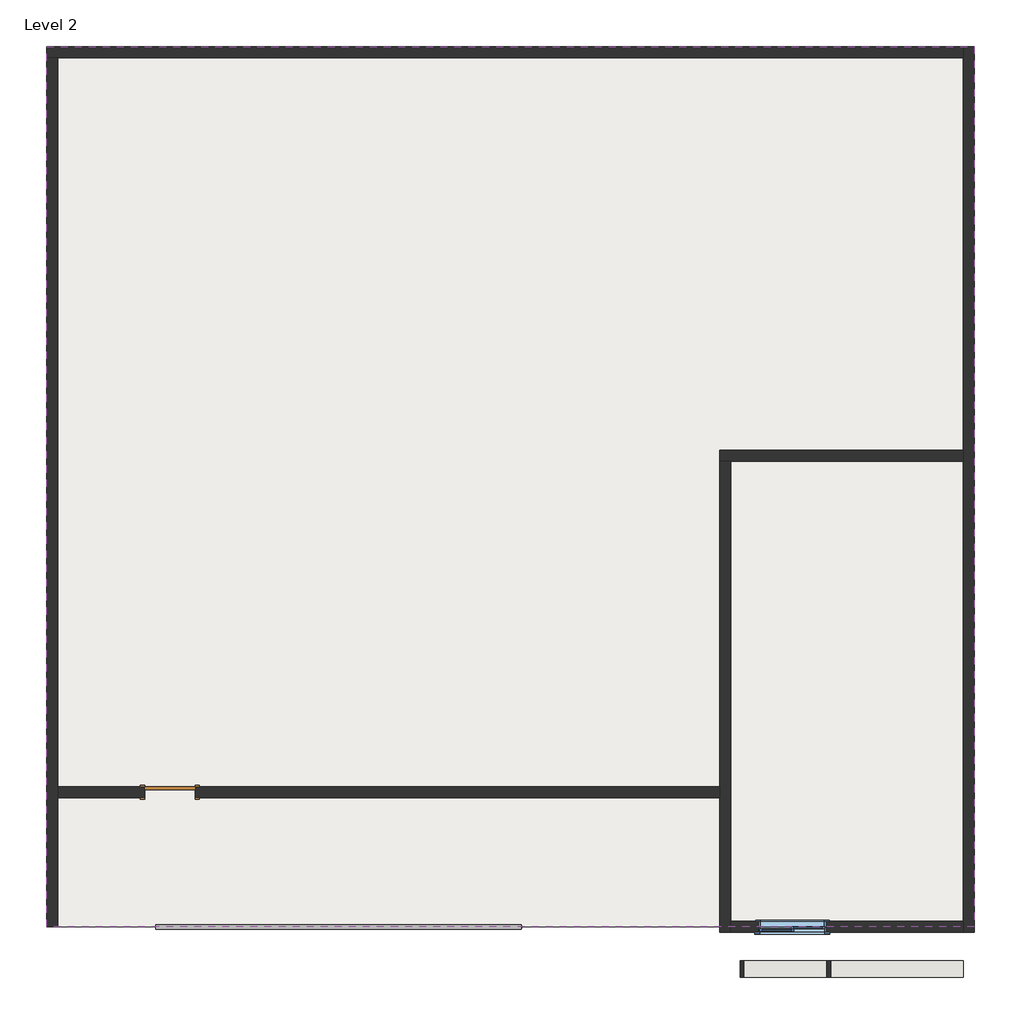
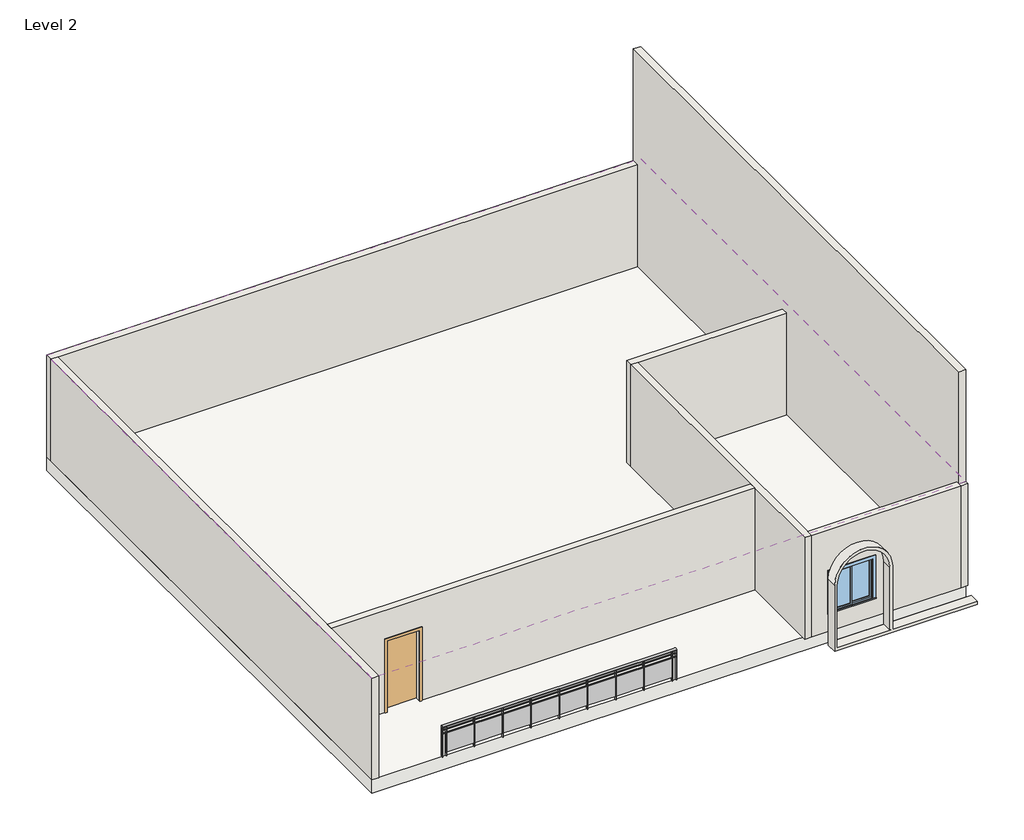
# One storey: 8 walls, 1 covering, 1 door, 1 railing, 1 slab, 1 window.
"""IFC4 building model written with IfcOpenShell, lengths in millimetres."""

from ifc_helpers import new_model, si_unit, point, frame, origin, place, context, project, spatial, polyline, ellipse_curve, trimmed, outline, extrude, faceted_brep, transform, mapped, element, save
from ifc_brep_helpers import plane_surface, extruded_surface, advanced_brep
from components import m_single_flush_0915_x_2134mm_727434cd, walls_5_walls_5_0e1fe4ca, window_deda82dd

model = new_model("IFC4")

# Units and contexts
model_context = context("Model", 3, world=origin())
ifc_project = project(units=[si_unit("LENGTHUNIT", "METRE", prefix="MILLI")], contexts=[model_context])

# Site, building, storey
site = spatial("IfcSite", under=ifc_project)
building = spatial("IfcBuilding", under=site)
storey = spatial("IfcBuildingStorey", under=building, Name="Level 2", Elevation=6096.0)

# Covering
placement = place(None, origin())
element("IfcCovering", 1, ObjectType="600 x 1200mm grid", at=placement, inside=storey, context=model_context, shape_type="SweptSolid", body=[
    extrude(outline(polyline([(-9031.8352527, 15360.4148445), (7778.3159626, 15360.4148445), (7778.3159626, -589.1851555), (-9031.8352527, -589.1851555), (-9031.8352527, 15360.4148445)])), frame((0.0, 0.0, 9144.0), z_axis=(0.0, 0.0, 1.0), x_axis=(1.0, 0.0, 0.0)), (0.0, 0.0, 1.0), 52.0),
])

# Door
m_single_flush_0915_x_2134mm_shape = m_single_flush_0915_x_2134mm_727434cd(model_context)
element("IfcDoor", 2, ObjectType="M_Single-Flush : 0915 x 2134mm", at=placement, inside=storey, context=model_context, shape_type="MappedRepresentation", body=[
    mapped(m_single_flush_0915_x_2134mm_shape, transform((-6798.2352527, 1849.2148445, 6096.0), x_axis=(-1.0, 0.0, 0.0), y_axis=(0.0, -1.0, 0.0), z_axis=(0.0, 0.0, 1.0))),
])

# Railing
element("IfcRailing", 3, ObjectType="Glass Panel - Bottom Fill", at=placement, inside=storey, context=model_context, shape_type="SolidModel", body=[
    advanced_brep(
    [(-7050.6352527, -549.7943903, 6996.0), (-7050.6352527, -629.7943903, 6996.0), (-429.4748459, -549.7943903, 6996.0), (-429.4748459, -629.7943903, 6996.0)],
    [
        (0, 1, ellipse_curve(frame((-7050.6352527, -589.7943903, 6996.0), z_axis=(-1.0, 0.0, 0.0), x_axis=(0.0, -1.0, 0.0)), 40.0, 30.0)),
        (1, 0, ellipse_curve(frame((-7050.6352527, -589.7943903, 6996.0), z_axis=(-1.0, 0.0, 0.0), x_axis=(0.0, -1.0, 0.0)), 40.0, 30.0)),
        (2, 3, ellipse_curve(frame((-429.4748459, -589.7943903, 6996.0), z_axis=(1.0, 0.0, 0.0), x_axis=(0.0, -1.0, 0.0)), 40.0, 30.0)),
        (3, 2, ellipse_curve(frame((-429.4748459, -589.7943903, 6996.0), z_axis=(1.0, 0.0, 0.0), x_axis=(0.0, -1.0, 0.0)), 40.0, 30.0)),
        (1, 3),
        (2, 0),
    ],
    [
        plane_surface(frame((-7050.6352527, -589.7943903, 6996.0), z_axis=(-1.0, 0.0, 0.0), x_axis=(0.0, 1.0, 0.0))),
        plane_surface(frame((-429.4748459, -589.7943903, 6996.0), z_axis=(1.0, 0.0, 0.0), x_axis=(0.0, 1.0, 0.0))),
        extruded_surface(trimmed(ellipse_curve(frame((-429.4748459, -589.7943903, 6996.0), z_axis=(-1.0, 0.0, 0.0), x_axis=(0.0, -1.0, 0.0)), 40.0, 30.0), [point((-429.4748459, -629.7943903, 6996.0))], [point((-429.4748459, -549.7943903, 6996.0))], True, "CARTESIAN"), (-6621.1604068, 0.0, 0.0), 6621.1604068),
        extruded_surface(trimmed(ellipse_curve(frame((-429.4748459, -589.7943903, 6996.0), z_axis=(-1.0, 0.0, 0.0), x_axis=(0.0, -1.0, 0.0)), 40.0, 30.0), [point((-429.4748459, -549.7943903, 6996.0))], [point((-429.4748459, -629.7943903, 6996.0))], True, "CARTESIAN"), (-6621.1604068, 0.0, 0.0), 6621.1604068),
    ],
    [
        (0, [[1, 2]]),
        (1, [[3, 4]]),
        (2, [[-2, 5, -3, 6]]),
        (3, [[-1, -6, -4, -5]]),
    ],
),
    extrude(outline(polyline([(-7050.6352527, -599.1851555), (-7050.6352527, -579.1851555), (-429.4748459, -579.1851555), (-429.4748459, -599.1851555), (-7050.6352527, -599.1851555)])), frame((0.0, 0.0, 6876.0), z_axis=(0.0, 0.0, 1.0), x_axis=(1.0, 0.0, 0.0)), (0.0, 0.0, 1.0), 20.0),
    extrude(outline(polyline([(-7050.6352527, -599.1851555), (-7050.6352527, -579.1851555), (-429.4748459, -579.1851555), (-429.4748459, -599.1851555), (-7050.6352527, -599.1851555)])), frame((0.0, 0.0, 6776.0), z_axis=(0.0, 0.0, 1.0), x_axis=(1.0, 0.0, 0.0)), (0.0, 0.0, 1.0), 20.0),
    extrude(outline(polyline([(-546.0550493, -564.1851555), (-534.0550493, -564.1851555), (-534.0550493, -614.1851555), (-546.0550493, -614.1851555), (-546.0550493, -564.1851555)])), frame((0.0, 0.0, 6096.0), z_axis=(0.0, 0.0, 1.0), x_axis=(1.0, 0.0, 0.0)), (0.0, 0.0, 1.0), 869.8465326),
    extrude(outline(polyline([(-1340.0550493, -590.9099656), (-540.0550493, -590.9099656), (-540.0550493, -595.9099656), (-1340.0550493, -595.9099656), (-1340.0550493, -590.9099656)])), frame((0.0, 0.0, 6196.0), z_axis=(0.0, 0.0, 1.0), x_axis=(1.0, 0.0, 0.0)), (0.0, 0.0, 1.0), 580.0),
    extrude(outline(polyline([(-1346.0550493, -564.1851555), (-1334.0550493, -564.1851555), (-1334.0550493, -614.1851555), (-1346.0550493, -614.1851555), (-1346.0550493, -564.1851555)])), frame((0.0, 0.0, 6096.0), z_axis=(0.0, 0.0, 1.0), x_axis=(1.0, 0.0, 0.0)), (0.0, 0.0, 1.0), 869.8465326),
    extrude(outline(polyline([(-2140.0550493, -590.9099656), (-1340.0550493, -590.9099656), (-1340.0550493, -595.9099656), (-2140.0550493, -595.9099656), (-2140.0550493, -590.9099656)])), frame((0.0, 0.0, 6196.0), z_axis=(0.0, 0.0, 1.0), x_axis=(1.0, 0.0, 0.0)), (0.0, 0.0, 1.0), 580.0),
    extrude(outline(polyline([(-2146.0550493, -564.1851555), (-2134.0550493, -564.1851555), (-2134.0550493, -614.1851555), (-2146.0550493, -614.1851555), (-2146.0550493, -564.1851555)])), frame((0.0, 0.0, 6096.0), z_axis=(0.0, 0.0, 1.0), x_axis=(1.0, 0.0, 0.0)), (0.0, 0.0, 1.0), 869.8465326),
    extrude(outline(polyline([(-2940.0550493, -590.9099656), (-2140.0550493, -590.9099656), (-2140.0550493, -595.9099656), (-2940.0550493, -595.9099656), (-2940.0550493, -590.9099656)])), frame((0.0, 0.0, 6196.0), z_axis=(0.0, 0.0, 1.0), x_axis=(1.0, 0.0, 0.0)), (0.0, 0.0, 1.0), 580.0),
    extrude(outline(polyline([(-2946.0550493, -564.1851555), (-2934.0550493, -564.1851555), (-2934.0550493, -614.1851555), (-2946.0550493, -614.1851555), (-2946.0550493, -564.1851555)])), frame((0.0, 0.0, 6096.0), z_axis=(0.0, 0.0, 1.0), x_axis=(1.0, 0.0, 0.0)), (0.0, 0.0, 1.0), 869.8465326),
    extrude(outline(polyline([(-3740.0550493, -590.9099656), (-2940.0550493, -590.9099656), (-2940.0550493, -595.9099656), (-3740.0550493, -595.9099656), (-3740.0550493, -590.9099656)])), frame((0.0, 0.0, 6196.0), z_axis=(0.0, 0.0, 1.0), x_axis=(1.0, 0.0, 0.0)), (0.0, 0.0, 1.0), 580.0),
    extrude(outline(polyline([(-3746.0550493, -564.1851555), (-3734.0550493, -564.1851555), (-3734.0550493, -614.1851555), (-3746.0550493, -614.1851555), (-3746.0550493, -564.1851555)])), frame((0.0, 0.0, 6096.0), z_axis=(0.0, 0.0, 1.0), x_axis=(1.0, 0.0, 0.0)), (0.0, 0.0, 1.0), 869.8465326),
    extrude(outline(polyline([(-4540.0550493, -590.9099656), (-3740.0550493, -590.9099656), (-3740.0550493, -595.9099656), (-4540.0550493, -595.9099656), (-4540.0550493, -590.9099656)])), frame((0.0, 0.0, 6196.0), z_axis=(0.0, 0.0, 1.0), x_axis=(1.0, 0.0, 0.0)), (0.0, 0.0, 1.0), 580.0),
    extrude(outline(polyline([(-4546.0550493, -564.1851555), (-4534.0550493, -564.1851555), (-4534.0550493, -614.1851555), (-4546.0550493, -614.1851555), (-4546.0550493, -564.1851555)])), frame((0.0, 0.0, 6096.0), z_axis=(0.0, 0.0, 1.0), x_axis=(1.0, 0.0, 0.0)), (0.0, 0.0, 1.0), 869.8465326),
    extrude(outline(polyline([(-5340.0550493, -590.9099656), (-4540.0550493, -590.9099656), (-4540.0550493, -595.9099656), (-5340.0550493, -595.9099656), (-5340.0550493, -590.9099656)])), frame((0.0, 0.0, 6196.0), z_axis=(0.0, 0.0, 1.0), x_axis=(1.0, 0.0, 0.0)), (0.0, 0.0, 1.0), 580.0),
    extrude(outline(polyline([(-5346.0550493, -564.1851555), (-5334.0550493, -564.1851555), (-5334.0550493, -614.1851555), (-5346.0550493, -614.1851555), (-5346.0550493, -564.1851555)])), frame((0.0, 0.0, 6096.0), z_axis=(0.0, 0.0, 1.0), x_axis=(1.0, 0.0, 0.0)), (0.0, 0.0, 1.0), 869.8465326),
    extrude(outline(polyline([(-6140.0550493, -590.9099656), (-5340.0550493, -590.9099656), (-5340.0550493, -595.9099656), (-6140.0550493, -595.9099656), (-6140.0550493, -590.9099656)])), frame((0.0, 0.0, 6196.0), z_axis=(0.0, 0.0, 1.0), x_axis=(1.0, 0.0, 0.0)), (0.0, 0.0, 1.0), 580.0),
    extrude(outline(polyline([(-6146.0550493, -564.1851555), (-6134.0550493, -564.1851555), (-6134.0550493, -614.1851555), (-6146.0550493, -614.1851555), (-6146.0550493, -564.1851555)])), frame((0.0, 0.0, 6096.0), z_axis=(0.0, 0.0, 1.0), x_axis=(1.0, 0.0, 0.0)), (0.0, 0.0, 1.0), 869.8465326),
    extrude(outline(polyline([(-6940.0550493, -590.9099656), (-6140.0550493, -590.9099656), (-6140.0550493, -595.9099656), (-6940.0550493, -595.9099656), (-6940.0550493, -590.9099656)])), frame((0.0, 0.0, 6196.0), z_axis=(0.0, 0.0, 1.0), x_axis=(1.0, 0.0, 0.0)), (0.0, 0.0, 1.0), 580.0),
    extrude(outline(polyline([(-6946.0550493, -564.1851555), (-6934.0550493, -564.1851555), (-6934.0550493, -614.1851555), (-6946.0550493, -614.1851555), (-6946.0550493, -564.1851555)])), frame((0.0, 0.0, 6096.0), z_axis=(0.0, 0.0, 1.0), x_axis=(1.0, 0.0, 0.0)), (0.0, 0.0, 1.0), 869.8465326),
    extrude(outline(polyline([(-437.4748459, -564.1851555), (-425.4748459, -564.1851555), (-425.4748459, -614.1851555), (-437.4748459, -614.1851555), (-437.4748459, -564.1851555)])), frame((0.0, 0.0, 6096.0), z_axis=(0.0, 0.0, 1.0), x_axis=(1.0, 0.0, 0.0)), (0.0, 0.0, 1.0), 869.8465326),
    extrude(outline(polyline([(-7054.6352527, -564.1851555), (-7042.6352527, -564.1851555), (-7042.6352527, -614.1851555), (-7054.6352527, -614.1851555), (-7054.6352527, -564.1851555)])), frame((0.0, 0.0, 6096.0), z_axis=(0.0, 0.0, 1.0), x_axis=(1.0, 0.0, 0.0)), (0.0, 0.0, 1.0), 869.8465326),
])

# Slab
element("IfcSlab", 4, ObjectType="Generic Floor - 400mm", at=placement, inside=storey, context=model_context, shape_type="SweptSolid", body=[
    extrude(outline(polyline([(-9031.8352527, 15360.4148445), (7778.3159626, 15360.4148445), (7778.3159626, -589.1851555), (-9031.8352527, -589.1851555), (-9031.8352527, 15360.4148445)])), frame((0.0, 0.0, 5696.0), z_axis=(0.0, 0.0, 1.0), x_axis=(1.0, 0.0, 0.0)), (0.0, 0.0, 1.0), 400.0),
])

# Walls
element("IfcWall", 5, ObjectType="Generic - 9\"", at=placement, inside=storey, context=model_context, shape_type="Brep", body=[
    faceted_brep([(-9031.8352527, 15160.4148445, 6096.0), (-8831.8352527, 15160.4148445, 6096.0), (7578.3159626, 15160.4148445, 6096.0), (7578.3159626, 15160.4148445, 9144.0), (-8831.8352527, 15160.4148445, 9144.0), (-9031.8352527, 15160.4148445, 9144.0), (-9031.8352527, 15360.4148445, 6096.0), (-9031.8352527, 15360.4148445, 9144.0), (7578.3159626, 15360.4148445, 9144.0), (7578.3159626, 15360.4148445, 6096.0)], [[[0, 1, 2, 3, 4, 5]], [[6, 7, 8, 9]], [[2, 1, 0, 6, 9]], [[5, 4, 3, 8, 7]], [[0, 5, 7, 6]], [[3, 2, 9, 8]]]),
])
element("IfcWall", 6, ObjectType="Generic - 9\"", at=placement, inside=storey, context=model_context, shape_type="Brep", body=[
    faceted_brep([(-8831.8352527, -589.1851555, 6096.0), (-8831.8352527, 1749.2148445, 6096.0), (-8831.8352527, 1949.2148445, 6096.0), (-8831.8352527, 15160.4148445, 6096.0), (-8831.8352527, 15160.4148445, 9144.0), (-8831.8352527, 1949.2148445, 9144.0), (-8831.8352527, 1749.2148445, 9144.0), (-8831.8352527, -589.1851555, 9144.0), (-9031.8352527, -589.1851555, 6096.0), (-9031.8352527, -589.1851555, 9144.0), (-9031.8352527, 15160.4148445, 9144.0), (-9031.8352527, 15160.4148445, 6096.0)], [[[0, 1, 2, 3, 4, 5, 6, 7]], [[8, 9, 10, 11]], [[3, 2, 1, 0, 8, 11]], [[7, 6, 5, 4, 10, 9]], [[0, 7, 9, 8]], [[4, 3, 11, 10]]]),
])
element("IfcWall", 7, ObjectType="Generic - 9\"", at=placement, inside=storey, context=model_context, shape_type="Brep", body=[
    faceted_brep([(7578.3159626, 15360.4148445, 6096.0), (7578.3159626, 15160.4148445, 6096.0), (7578.3159626, 8045.2148445, 6096.0), (7578.3159626, 7845.2148445, 6096.0), (7578.3159626, -489.1851555, 6096.0), (7578.3159626, -689.1851555, 6096.0), (7578.3159626, -689.1851555, 9144.0), (7578.3159626, -589.1851555, 9144.0), (7578.3159626, -589.1851555, 12496.8), (7578.3159626, 15360.4148445, 12496.8), (7578.3159626, 15360.4148445, 9144.0), (7778.3159626, 15360.4148445, 6096.0), (7778.3159626, 15360.4148445, 12496.8), (7778.3159626, -589.1851555, 12496.8), (7778.3159626, -589.1851555, 9144.0), (7778.3159626, -689.1851555, 9144.0), (7778.3159626, -689.1851555, 6096.0)], [[[0, 1, 2, 3, 4, 5, 6, 7, 8, 9, 10]], [[11, 12, 13, 14, 15, 16]], [[5, 4, 3, 2, 1, 0, 11, 16]], [[9, 8, 13, 12]], [[0, 10, 9, 12, 11]], [[8, 7, 14, 13]], [[14, 7, 6, 15]], [[6, 5, 16, 15]]]),
])
element("IfcWall", 8, ObjectType="Generic - 9\"", at=placement, inside=storey, context=model_context, shape_type="Brep", body=[
    faceted_brep([(3160.1647473, 7845.2148445, 6096.0), (3360.1647473, 7845.2148445, 6096.0), (7578.3159626, 7845.2148445, 6096.0), (7578.3159626, 7845.2148445, 9144.0), (3360.1647473, 7845.2148445, 9144.0), (3160.1647473, 7845.2148445, 9144.0), (3160.1647473, 8045.2148445, 6096.0), (3160.1647473, 8045.2148445, 9144.0), (7578.3159626, 8045.2148445, 9144.0), (7578.3159626, 8045.2148445, 6096.0)], [[[0, 1, 2, 3, 4, 5]], [[6, 7, 8, 9]], [[2, 1, 0, 6, 9]], [[5, 4, 3, 8, 7]], [[0, 5, 7, 6]], [[3, 2, 9, 8]]]),
])
element("IfcWall", 9, ObjectType="Generic - 9\"", at=placement, inside=storey, context=model_context, shape_type="Brep", body=[
    faceted_brep([(3360.1647473, -689.1851555, 6096.0), (3360.1647473, -489.1851555, 6096.0), (3360.1647473, 7845.2148445, 6096.0), (3360.1647473, 7845.2148445, 9144.0), (3360.1647473, -489.1851555, 9144.0), (3360.1647473, -689.1851555, 9144.0), (3160.1647473, -689.1851555, 6096.0), (3160.1647473, -689.1851555, 9144.0), (3160.1647473, 1749.2148445, 9144.0), (3160.1647473, 1949.2148445, 9144.0), (3160.1647473, 7845.2148445, 9144.0), (3160.1647473, 7845.2148445, 6096.0), (3160.1647473, 1949.2148445, 6096.0), (3160.1647473, 1749.2148445, 6096.0)], [[[0, 1, 2, 3, 4, 5]], [[6, 7, 8, 9, 10, 11, 12, 13]], [[2, 1, 0, 6, 13, 12, 11]], [[5, 4, 3, 10, 9, 8, 7]], [[3, 2, 11, 10]], [[0, 5, 7, 6]]]),
])
element("IfcWall", 10, ObjectType="Generic - 9\"", at=placement, inside=storey, context=model_context, shape_type="SweptSolid", body=[
    extrude(outline(polyline([(6096.0, -8831.8352527), (6096.0, -7255.7352527), (8230.0, -7255.7352527), (8230.0, -6340.7352527), (6096.0, -6340.7352527), (6096.0, 3160.1647473), (9144.0, 3160.1647473), (9144.0, -8831.8352527), (6096.0, -8831.8352527)])), frame((0.0, 1749.2148445, 0.0), z_axis=(0.0, 1.0, 0.0), x_axis=(0.0, 0.0, 1.0)), (0.0, 0.0, 1.0), 200.0),
])
element("IfcWall", 11, ObjectType="Generic - 9\"", at=placement, inside=storey, context=model_context, shape_type="Brep", body=[
    faceted_brep([(3360.1647473, -689.1851555, 6096.0), (7578.3159626, -689.1851555, 6096.0), (7578.3159626, -689.1851555, 9144.0), (3360.1647473, -689.1851555, 9144.0), (3869.7647473, -689.1851555, 7865.6356792), (5088.9647473, -689.1851555, 7865.6356792), (5088.9647473, -689.1851555, 6646.4356792), (3869.7647473, -689.1851555, 6646.4356792), (3360.1647473, -489.1851555, 6096.0), (3360.1647473, -489.1851555, 9144.0), (7578.3159626, -489.1851555, 9144.0), (7578.3159626, -489.1851555, 6096.0), (3869.7647473, -489.1851555, 7865.6356792), (3869.7647473, -489.1851555, 6646.4356792), (5088.9647473, -489.1851555, 6646.4356792), (5088.9647473, -489.1851555, 7865.6356792), (7578.3159626, -589.1851555, 9144.0)], [[[0, 1, 2, 3], [4, 5, 6, 7]], [[8, 9, 10, 11], [12, 13, 14, 15]], [[1, 0, 8, 11]], [[3, 2, 16, 10, 9]], [[0, 3, 9, 8]], [[2, 1, 11, 10, 16]], [[13, 12, 4, 7]], [[14, 13, 7, 6]], [[15, 14, 6, 5]], [[12, 15, 5, 4]]]),
])
walls_5_walls_5_shape = walls_5_walls_5_0e1fe4ca(model_context)
element("IfcWall", 12, ObjectType="Walls 5 : Walls 5", at=placement, inside=storey, context=model_context, shape_type="MappedRepresentation", body=[
    mapped(walls_5_walls_5_shape, transform((0.0, 0.0, 0.0), x_axis=(1.0, 0.0, 0.0), y_axis=(0.0, 1.0, 0.0), z_axis=(0.0, 0.0, 1.0))),
])

# Window
window_shape = window_deda82dd(model_context)
element("IfcWindow", 13, ObjectType="Slider with Trim : 48\" x 48\"", at=placement, inside=storey, context=model_context, shape_type="MappedRepresentation", body=[
    mapped(window_shape, transform((4479.3647473, -589.1851555, 5732.0356792), x_axis=(-1.0, 0.0, 0.0), y_axis=(0.0, -1.0, 0.0), z_axis=(0.0, 0.0, 1.0))),
])

save(model, "model.ifc")

# Revit data of these elements
# Type "600 x 1200mm grid"
#   built-in parameter 1002203 = 1 (stored number, unit not read)
#   built-in parameter 1002202 = 1 (stored number, unit not read)
#   Layers, outside or top first: 0' - 1.41732" "Default" (function 1); 0' - 0.62992" "Ceiling Tile 600 x 1200" (function 5)
# Type "M_Single-Flush : 0915 x 2134mm"
#   Type Mark = "15"
#   Thickness = 0' - 2.00787"
#   Height = 7' - 0.01575"
#   Trim Projection Ext = 0' - 0.98425"
#   Trim Projection Int = 0' - 0.98425"
#   Trim Width = 0' - 2.99213"
#   Width = 3' - 0.02362"
#   Door Material = Door - Panel
#   Frame Material = Door - Frame
#   Function = (empty or 0)
#   Wall Closure = (empty or 0)
# Type "Glass Panel - Bottom Fill"
#   built-in parameter 1008612 = 0.019685 (stored number, unit not read)
#   built-in parameter 1008611 = 0.019685 (stored number, unit not read)
#   built-in parameter 1008609 = 0.902231 (stored number, unit not read)
#   built-in parameter 1008604 = 0.19685 (stored number, unit not read)
#   built-in parameter 1008603 = 0.164042 (stored number, unit not read)
#   Railing Height = 2' - 11.43307"
#   built-in parameter 1008630 = 2
#   built-in parameter 1008610 = 2
# Type "Generic Floor - 400mm"
#   Function = 0
#   Layers, outside or top first: 1' - 3.74803" no material (function 1)
# Type "Generic - 9\""
#   Layers, outside or top first: 0' - 7.87402" no material (function 1)
# Type "Slider with Trim : 48\" x 48\""
#   Type Mark = "24"
#   Construction Type Id = "GSP4R"
#   Assembly Code = "B2020100"
#   Analytic Construction = "1/8 in Pilkington single glazing"
#   Visual Light Transmittance = 0.9
#   Solar Heat Gain Coefficient = 0.78
#   Heat Transfer Coefficient (U) = 3.6886 W/(m²·K)
#   Height = 4' - 0"
#   Default Sill Height = 3' - 0"
#   Trim Projection - Ext. = 0' - 0 3/4"
#   Trim Projection - Int. = 0' - 0 3/4"
#   Trim Width - Exterior = 0' - 3 1/2"
#   Trim Width - Interior = 0' - 3 1/2"
#   Width = 4' - 0"
#   Window Inset = 0' - 0 3/4"
#   Define Thermal Properties by = 1
#   Glass Pane Material = Glass
#   Sash Material = Sash
#   Trim Exterior Material = Trim
#   Trim Interior Material = Trim
#   Wall Closure = (empty or 0)
# Element 1 (IfcCovering, "600 x 1200mm grid")
#   Height Offset From Level = 10' - 0"
#   Phase Created = New Construction
#   Materials on its faces: "Ceiling Tile 600 x 1200", "Default"
# Element 2 (IfcDoor, "M_Single-Flush : 0915 x 2134mm")
#   Phase Created = New Construction
#   Materials on its faces: "Door - Frame", "Door - Panel"
# Element 3 (IfcRailing, "Glass Panel - Bottom Fill")
#   Phase Created = New Construction
#   Materials on its faces: "Metal - Stainless Steel,Polished", "Glass"
# Element 4 (IfcSlab, "Generic Floor - 400mm")
#   built-in parameter 1001955 = 3.14159 (stored number, unit not read)
#   Height Offset From Level = 0' - 0"
#   Phase Created = New Construction
#   Materials on its faces: "Default Roof"
# Elements 5, 6, 8, 9, 10, 11 (IfcWall, "Generic - 9\"")
#   Top Offset = 0' - 0"
#   Base Offset = 0' - 0"
#   Unconnected Height = 10' - 0"
#   wall height = 10' - 0"
#   Phase Created = New Construction
#   Base Constraint = Level 2
#   Materials on its faces: "Default Wall"
# Element 7 (IfcWall, "Generic - 9\"")
#   Top Offset = 0' - 0"
#   Base Offset = 0' - 0"
#   Unconnected Height = 21' - 0"
#   wall height = 21' - 0"
#   Phase Created = New Construction
#   Base Constraint = Level 2
#   Materials on its faces: "Default Wall"
# Element 12 (IfcWall, "Walls 5 : Walls 5")
#   Phase Created = New Construction
#   Materials on its faces: "Default Wall"
# Element 13 (IfcWindow, "Slider with Trim : 48\" x 48\"")
#   Mark = "13"
#   Phase Created = New Construction
#   Materials on its faces: "Sash", "Trim", "Glass"
# Materials
#   "Default": colour RGB 80 80 80, transparency 0
#   "Ceiling Tile 600 x 1200": class "Generic", colour RGB 179 178 175, transparency 0, Description = "Acoustic ceiling tile", Cost = 0
#   "Door - Panel": class "Wood", colour RGB 114 82 51, transparency 0
#   "Door - Frame": colour RGB 153 76 43, transparency 0
#   "Glass": class "Glass", colour RGB 218 227 224, transparency 0.85, Description = "Soda Lime Glass", Cost = 0
#   "Sash": class "Wood", colour RGB 136 99 55, transparency 0
#   "Trim": class "Wood", colour RGB 224 178 126, transparency 0
#   "Metal - Stainless Steel,Polished": class "Metal", colour RGB 189 187 185, transparency 0, Cost = 0
#   "Default Roof": colour RGB 80 80 80, transparency 0
#   "Default Wall": colour RGB 80 80 80, transparency 0
